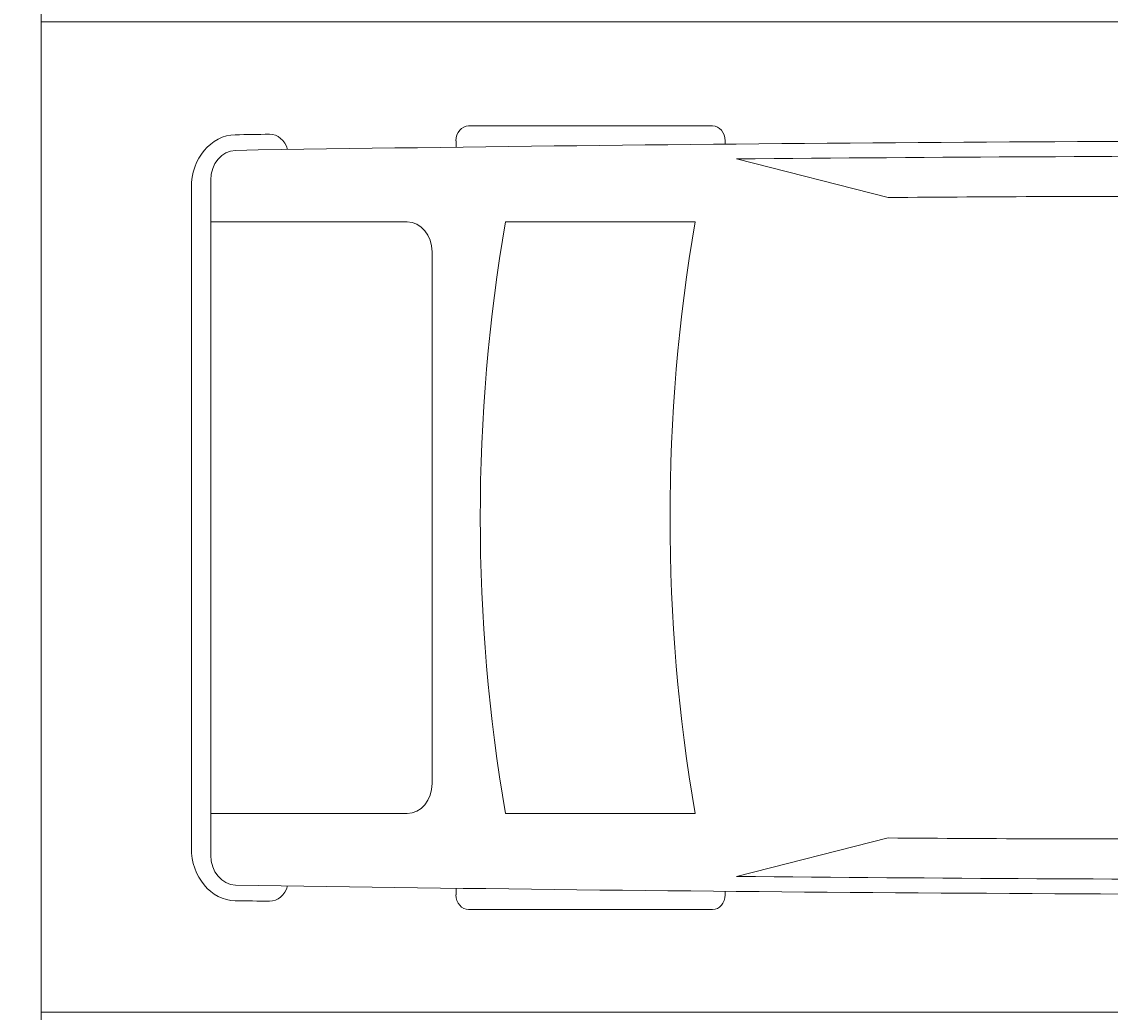
# Model space of a CAD drawing. Units: inches. Extents: x -46 to 1145, y -527 to 760.
# Tile 9 of 57: x 272 to 380, y -270 to -172. Entities that reach past the tile are written whole.
import ezdxf

# ---------------------------------------------------------------- set-up
doc = ezdxf.new("R2010")
doc.units = ezdxf.units.IN
doc.header["$MEASUREMENT"] = 0
for name, color, linetype, lineweight in [('A-ANNO-DIMS', 2, 'Continuous', 18), ('C-PKNG', 8, 'Continuous', 18), ('C-PKNG-VEHI', 8, 'Continuous', 13)]:
    doc.layers.add(name, color=color, linetype=linetype, lineweight=lineweight)
doc.styles.get("Standard").update_dxf_attribs({"font": 'arial.ttf'})
doc.dimstyles.get("Standard").update_dxf_attribs({"dimtxt": 0.18, "dimasz": 0.18, "dimexe": 0.18, "dimexo": 0.0625, "dimgap": 0.09, "dimtad": 0, "dimtih": 1, "dimtoh": 1, "dimdec": 0, "dimzin": 0, "dimdsep": 46, "dimlunit": 3, "dimtxsty": 'Standard', "dimcen": 0.09, "dimadec": 0, "dimazin": 0, "dimtfac": 1, "dimtdec": 0, "dimtofl": 0, "dimtmove": 0, "dimatfit": 3, "dimfxl": 1, "dimtolj": 1, "dimtzin": 0, "dimarcsym": 0})

# ---------------------------------------------------------------- blocks, each defined once
blk = doc.blocks.new('*U640')
for p, q in [((1182.5, 987.8), (567.7, 987.8)), ((3472.1, 987.8), (4086.9, 987.8)), ((536, 950.2), (536, 935.5)), ((1214.1, 949.7), (1214.1, 950.2)), ((3440.5, 941.7), (3440.5, 950.2)), ((4118.5, 950.2), (4118.5, 934.1)), ((2234.8, 809.5), (1898.9, 912.4)), ((3411.6, 904.3), (3029.9, 807.2)), ((4736.4, -850.9), (4736.4, 850.9)), ((4785.3, -832.1), (4785.3, 832.1)), ((1778.8, 801), (2194.7, 745.5)), ((3515.9, 745.5), (3994.1, 745.5)), ((4736.4, 745.5), (4242, 745.5)), ((4178.7, 670.3), (4178.7, -670.3)), ((819.6, 295.3), (917.7, 436.1)), ((917.7, 436.1), (1293.8, 436.1)), ((815.9, 241.4), (815.9, 283.3)), ((1496.5, -273.7), (1496.5, 273.7)), ((1690.4, -267.4), (1690.4, 267.4)), ((4736.4, -267.4), (4736.4, 267.4)), ((756.2, 241.4), (1312.8, 241.4)), ((2101.5, 215.8), (2101.5, -215.8)), ((83, 155.7), (2.6, 10.3)), ((0, 0), (1312.8, 0)), ((2.6, -10.3), (83, -155.7)), ((756.2, -241.4), (1312.8, -241.4)), ((815.9, -241.4), (815.9, -283.3)), ((819.6, -295.3), (917.7, -436.1)), ((917.7, -436.1), (1293.8, -436.1)), ((2194.7, -745.5), (1778.8, -801)), ((3994.1, -745.5), (3515.9, -745.5)), ((4242, -745.5), (4736.4, -745.5)), ((2234.8, -809.5), (1898.9, -912.4)), ((3411.6, -904.3), (3029.9, -807.2)), ((536, -950.2), (536, -935.5)), ((1214.1, -949.7), (1214.1, -950.2)), ((3440.5, -941.7), (3440.5, -950.2)), ((4118.5, -950.2), (4118.5, -934.1)), ((1182.5, -987.8), (567.7, -987.8)), ((3472.1, -987.8), (4086.9, -987.8))]:
    blk.add_line(p, q)
for centre, major_axis, ratio, start_param, end_param in [((567.7, 950.2), (0, -37.6), 0.842304, 3.141593, 4.712389), ((1182.5, 950.2), (0, 37.6), 0.842304, -1.570796, 0), ((3472.1, 950.2), (0, -37.6), 0.842304, 3.141593, 4.712389), ((4086.9, 950.2), (0, 37.6), 0.842304, -1.570796, 0), ((4588, 910.3), (0, 56.4), 0.842304, -0.013017, 1.249894), ((1637.8, -268131.5), (0, 269121), 0.842304, -0.013397, -0.013017), ((4673.1, 832.1), (0, -133.3), 0.842304, 1.570796, 3.128196), ((1046.3, -12467.9), (0, 13417.1), 0.842304, 0.00281, 0.075598), ((1637.8, -268112.7), (0, 269062.9), 0.842304, -0.013397, 0.002797), ((6757.2, -699.1), (0, 7958), 0.842304, 1.367076, 1.39176), ((1637.8, -268112.7), (0, -269025.3), 0.842304, 3.133765, 3.140441), ((4673.1, 850.9), (0, -75.2), 0.842304, 1.570796, 3.128196), ((3436.4, 136.8), (0, 2077), 0.842304, 1.245306, 1.50788), ((2433, -93125.4), (0, -93935.2), 0.842304, 3.134049, 3.144098), ((951.8, -15086.6), (0, -15832.5), 0.842304, 3.096046, 3.200911), ((3799.7, 71.1), (0, -2021.3), 0.842304, 4.372215, 4.640744), ((433.9, 0), (0, 3734.3), 0.842304, 4.511394, 4.913384), ((912, 0), (0, 3734.3), 0.842304, 4.511394, 4.913384), ((4242, 670.3), (0, 75.2), 0.842304, 0, 1.570796), ((6583, -699.1), (0, -7754.7), 0.842304, 4.528606, 4.561838), ((3413.8, 136.8), (0, -2280.3), 0.842304, 4.449482, 4.652344), ((-5194.2, 1330.9), (0, -6374.4), 0.842304, 1.385369, 1.434372), ((331.1, 432), (0, 696.4), 0.842304, 4.435146, 4.718221), ((360.7, 432), (0, 696.4), 0.842304, 4.435146, 4.718221), ((1290.1, 338.8), (161, -9.1), 0.603834, -1.395552, 1.581315), ((831.8, 283.3), (0, 18.8), 0.842304, 0.879714, 1.570796), ((756.2, -1185.2), (0, 1426.7), 0.842304, 0, 0.590319), ((15.8, 0), (0, -18.8), 0.842304, 4.131459, 5.293319), ((756.2, 1185.2), (0, 1426.7), 0.842304, 2.551274, 3.141593), ((-5194.2, -1330.9), (0, 6374.4), 0.842304, -1.434372, -1.385369), ((3799.7, -71.1), (0, -2021.3), 0.842304, -1.499151, -1.230623), ((331.1, -432), (0, -696.4), 0.842304, 1.564964, 1.848039), ((360.7, -432), (0, -696.4), 0.842304, 1.564964, 1.848039), ((3413.8, -136.8), (0, -2280.3), 0.842304, -1.510751, -1.307889), ((3436.4, -136.8), (0, -2077), 0.842304, -1.50788, -1.245306), ((831.8, -283.3), (0, -18.8), 0.842304, 4.712389, 5.403472), ((6583, 699.1), (0, 7754.7), 0.842304, 1.721348, 1.754579), ((4242, -670.3), (0, -75.2), 0.842304, 4.712389, 6.283185), ((6757.2, 699.1), (0, 7958), 0.842304, 1.749832, 1.774517), ((951.8, 15086.6), (0, -15832.5), 0.842304, -0.059319, 0.045547), ((2433, 93125.4), (0, -93935.2), 0.842304, -0.002505, 0.007544), ((4673.1, -832.1), (0, -133.3), 0.842304, 0.013397, 1.570796), ((4673.1, -850.9), (0, 75.2), 0.842304, 3.15499, 4.712389), ((1637.8, 268112.7), (0, -269025.3), 0.842304, 0.001152, 0.007828), ((1046.3, 12467.9), (0, -13417.1), 0.842304, -0.075598, -0.00281), ((1637.8, 268112.7), (0, 269062.9), 0.842304, 3.138796, 3.15499), ((4588, -910.3), (0, -56.4), 0.842304, -1.249894, 0.013017), ((567.7, -950.2), (0, 37.6), 0.842304, 1.570796, 3.141593), ((1182.5, -950.2), (0, -37.6), 0.842304, 0, 1.570796), ((3472.1, -950.2), (0, -37.6), 0.842304, -1.570796, 0), ((4086.9, -950.2), (0, 37.6), 0.842304, 3.141593, 4.712389), ((1637.8, 268131.5), (0, 269121), 0.842304, 3.15461, 3.15499)]:
    blk.add_ellipse(centre, major_axis=major_axis, ratio=ratio, start_param=start_param, end_param=end_param)
at = {"extrusion": (0, 0, -1)}
blk.add_ellipse((1290.1, -338.8), major_axis=(161, 9.1), ratio=0.603834, start_param=-1.395552, end_param=1.581315, dxfattribs=at)
blk = doc.blocks.new('*D702')
at = {"layer": 'A-ANNO-DIMS', "color": 0, "lineweight": -2, "transparency": 16777216}
for p, q in [((189.63, -39.48), (1145.34, -39.48)), ((1145.16, -39.66), (1145.16, -249.3)), ((1145.16, -459.3), (1145.16, -249.66)), ((183.63, -459.48), (1145.34, -459.48))]:
    blk.add_line(p, q, dxfattribs=at)
at = {"layer": 'A-ANNO-DIMS', "color": 0, "transparency": 16777216}
for points in [[(1145.13, -39.66), (1145.19, -39.66), (1145.16, -39.48)], [(1145.13, -459.3), (1145.19, -459.3), (1145.16, -459.48)]]:
    blk.add_solid(points, dxfattribs=at)
at = {"layer": 'Defpoints', "color": 0, "transparency": 16777216}
for p in [(189.56, -39.48), (1145.16, -39.48), (183.56, -459.48)]:
    blk.add_point(p, dxfattribs=at)
at = {"layer": 'A-ANNO-DIMS', "color": 0, "transparency": 16777216, "insert": (1145.16, -249.48), "char_height": 0.18, "attachment_point": 5}
blk.add_mtext('\\A1;420', dxfattribs=at)

msp = doc.modelspace()

# ---------------------------------------------------------------- linework, layer by layer
at = {"layer": 'C-PKNG'}
msp.add_line((273.5156, -39.4824), (273.5156, -459.4824), dxfattribs=at)
msp.add_lwpolyline([(501.7297, -270.4792), (273.5156, -270.4792), (273.5156, -172.1813), (501.7297, -172.1813)], close=True, dxfattribs=at)

# ---------------------------------------------------------------- block references
at = {"layer": 'C-PKNG-VEHI', "xscale": 0.0393700787401575, "yscale": 0.0393700787401575, "zscale": 0.0393700787401575, "rotation": 180}
msp.add_blockref('*U640', (476.808, -221.4019), dxfattribs=at)

# ---------------------------------------------------------------- dimensions: what is measured, and where the dimension line sits
at = {"layer": 'A-ANNO-DIMS'}
dim = msp.add_linear_dim(base=(1145.1637, -39.4824), p1=(183.5637, -459.4824), p2=(189.5637, -39.4824), angle=90, dimstyle='Standard', override={"dimdec": 0, "dimlfac": 1, "dimrnd": 0, "dimzin": 0, "dimdsep": 46, "dimlunit": 2}, dxfattribs=at)
dim.commit()
dim.dimension.update_dxf_attribs({"geometry": '*D702', "text_midpoint": (1145.1637, -249.4824)})

doc.saveas('drawing.dxf')
